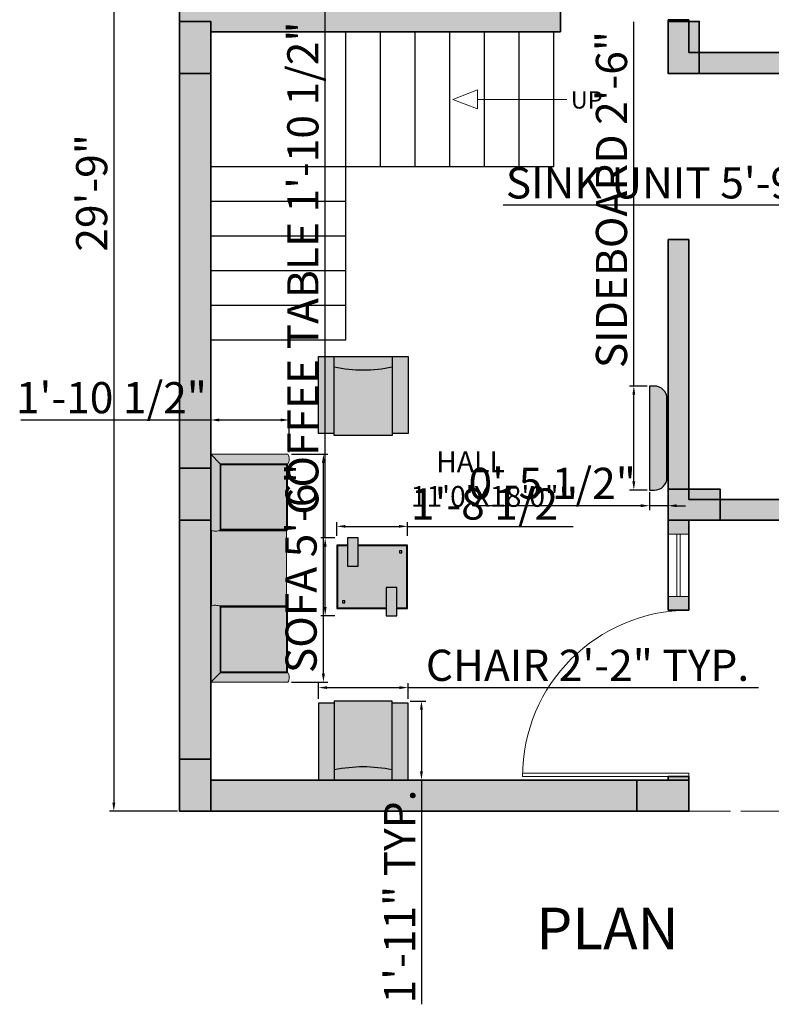
# Model space of a CAD drawing. Units: inches. Extents: x 3148 to 3962, y 1142 to 1671.
# Tile 1 of 9: x 3148 to 3365, y 1142 to 1426. Entities that reach past the tile are written whole.
import ezdxf

# ---------------------------------------------------------------- set-up
doc = ezdxf.new("R2010")
doc.units = ezdxf.units.IN
doc.linetypes.add('ACAD_ISO02W100', pattern=[15, 12, -3])
for name, color, linetype, lineweight in [('A-ANNO-DIMS', 2, 'Continuous', 18), ('A-ANNO-SYMB', 7, 'Continuous', 18), ('A-ANNO-TEXT', 7, 'Continuous', 25), ('A-AREA-IDEN', 7, 'Continuous', 18), ('A-COLS', 1, 'Continuous', 35), ('A-DOOR', 3, 'Continuous', 18), ('A-FLOR-STRS', 7, 'Continuous', 25), ('A-FURN', 8, 'Continuous', 18), ('A-GLAZ', 4, 'Continuous', 18), ('A-ROOF-OVHD', 7, 'ACAD_ISO02W100', 18), ('A-WALL', 7, 'Continuous', 35), ('moveis', 254, 'Continuous', 5), ('parede', 7, 'Continuous', 30)]:
    doc.layers.add(name, color=color, linetype=linetype, lineweight=lineweight)
doc.layers.add('A-WALL-PATT', color=252, linetype='Continuous', lineweight=13, true_color=0x939598)
doc.layers.add('MESA', color=7, linetype='Continuous')
doc.layers.add('MOBIL', color=7, linetype='Continuous')
doc.styles.get("Standard").update_dxf_attribs({"font": 'arial.ttf'})
doc.dimstyles.new('ISO-25', dxfattribs={"dimtxt": 9, "dimasz": 2.5, "dimexe": 1.25, "dimexo": 0.625, "dimtad": 1, "dimdec": 1, "dimlunit": 3, "dimtxsty": 'Standard', "dimcen": 2.5, "dimadec": 0, "dimazin": 0, "dimtfac": 1, "dimtdec": 1, "dimtmove": 0, "dimatfit": 3, "dimfxl": 1, "dimarcsym": 0})

# ---------------------------------------------------------------- blocks, each defined once
blk = doc.blocks.new('Poltrona Zoom Bolis')
at = {"layer": 'moveis'}
h = blk.add_hatch(color=256, dxfattribs=at)
h.set_gradient(color1=(102, 74, 66), color2=(156, 115, 104), one_color=1, tint=0.51)
h.paths.add_polyline_path([(-0.8363, -0.5604, 0.119368), (-0.805, -0.5689), (-0.7999, -0.5689, 0.109048), (-0.7663, -0.5612), (-0.7663, -0.0639), (-0.8363, 0.0061)])
h = blk.add_hatch(color=256, dxfattribs=at)
h.set_gradient(color1=(102, 74, 66), color2=(156, 115, 104), one_color=1, tint=0.51, name='INVCURVED')
h.paths.add_polyline_path([(-0.2778, -0.0639, 0.078404), (-0.2713, -0.0289), (-0.2713, -0.0252, 0.119368), (-0.2798, 0.0061), (-0.8363, 0.0061), (-0.7663, -0.0639)])
h.paths.add_polyline_path([(0.7663, -0.0639), (0.8363, 0.0061), (0.2798, 0.0061, 0.119368), (0.2713, -0.0252), (0.2713, -0.0289, 0.078404), (0.2778, -0.0639)])
h = blk.add_hatch(color=256, dxfattribs=at)
h.set_gradient(color1=(102, 74, 66), color2=(108, 79, 71), one_color=1, tint=0.35, name='CYLINDER')
h.paths.add_polyline_path([(-0.275, 0), (-0.275, -0.0047, -0.090212), (-0.2713, -0.029, -0.057138), (-0.275, -0.0548), (-0.275, -0.55), (0.275, -0.55), (0.275, -0.0548, -0.057138), (0.2713, -0.029, -0.090212), (0.275, -0.0047), (0.275, 0)])
h = blk.add_hatch(color=256, dxfattribs=at)
h.set_gradient(color1=(102, 74, 66), color2=(156, 115, 104), one_color=1, tint=0.51)
h.paths.add_polyline_path([(0.7663, -0.5612, 0.109048), (0.7999, -0.5689), (0.805, -0.5689, 0.119368), (0.8363, -0.5604), (0.8363, 0.0061), (0.7663, -0.0639)])
h = blk.add_hatch(color=256, dxfattribs=at)
h.set_gradient(color1=(102, 74, 66), color2=(96, 70, 62), one_color=1, tint=0.31, name='CYLINDER')
h.paths.add_polyline_path([(-0.7663, -0.0639), (-0.759, -0.0691), (-0.2798, -0.0691, 0.012038), (-0.2778, -0.0639)])
h.paths.add_polyline_path([(-0.759, -0.0691), (-0.7663, -0.0639), (-0.7663, -0.5612, 0.025931), (-0.759, -0.5573)])
h.paths.add_polyline_path([(-0.2804, -0.0691), (-0.2863, -0.0691), (-0.2863, -0.5489), (-0.759, -0.5489), (-0.759, -0.5573), (-0.2804, -0.5573)])
h = blk.add_hatch(color=256, dxfattribs=at)
h.set_gradient(color1=(102, 74, 66), color2=(156, 115, 104), one_color=1, tint=0.51, name='INVCYLINDER')
h.paths.add_polyline_path([(-0.759, -0.0691), (-0.759, -0.5489), (-0.2863, -0.5489), (-0.2863, -0.0691)])
h = blk.add_hatch(color=256, dxfattribs=at)
h.set_gradient(color1=(102, 74, 66), color2=(96, 70, 62), one_color=1, tint=0.31, name='CYLINDER')
h.paths.add_polyline_path([(0.7663, -0.0639), (0.2778, -0.0639, 0.012038), (0.2798, -0.0691), (0.759, -0.0691)])
h = blk.add_hatch(color=256, dxfattribs=at)
h.set_gradient(color1=(102, 74, 66), color2=(96, 70, 62), one_color=1, tint=0.31, name='CYLINDER')
h.paths.add_polyline_path([(0.2863, -0.0691), (0.2804, -0.0691), (0.2804, -0.5573), (0.759, -0.5573), (0.759, -0.5489), (0.2863, -0.5489)])
h = blk.add_hatch(color=256, dxfattribs=at)
h.set_gradient(color1=(102, 74, 66), color2=(156, 115, 104), one_color=1, tint=0.51, name='INVCYLINDER')
h.paths.add_polyline_path([(0.2863, -0.0691), (0.2863, -0.5489), (0.759, -0.5489), (0.759, -0.0691)])
h = blk.add_hatch(color=256, dxfattribs=at)
h.set_gradient(color1=(102, 74, 66), color2=(96, 70, 62), one_color=1, tint=0.31, name='CYLINDER')
h.paths.add_polyline_path([(0.759, -0.5573, 0.025931), (0.7663, -0.5612), (0.7663, -0.0639), (0.759, -0.0691)])
for p, q in [((-0.8363, 0.0061), (-0.8363, -0.5604)), ((-0.8363, 0.0061), (-0.2798, 0.0061)), ((-0.8363, 0.0061), (-0.7663, -0.0639)), ((0.275, 0), (-0.275, 0)), ((-0.275, -0.0047), (-0.275, 0)), ((0.275, -0.0047), (0.275, 0)), ((0.275, -0.0047), (0.275, 0)), ((0.8363, 0.0061), (0.2798, 0.0061)), ((0.8363, 0.0061), (0.7663, -0.0639)), ((0.8363, 0.0061), (0.8363, -0.5604)), ((-0.7663, -0.5612), (-0.7663, -0.0639)), ((-0.7663, -0.0639), (-0.2778, -0.0639)), ((-0.7663, -0.0639), (-0.759, -0.0691)), ((-0.759, -0.5573), (-0.759, -0.0691)), ((-0.759, -0.0691), (-0.2798, -0.0691)), ((-0.2863, -0.5489), (-0.2863, -0.0691)), ((-0.2804, -0.5573), (-0.2804, -0.0691)), ((-0.275, -0.55), (-0.275, -0.0548)), ((-0.2713, -0.0252), (-0.2713, -0.0327)), ((-0.2713, -0.0327), (-0.2713, -0.0252)), ((0.2713, -0.0252), (0.2713, -0.0327)), ((0.2713, -0.0327), (0.2713, -0.0252)), ((0.275, -0.55), (0.275, -0.0548)), ((0.7663, -0.0639), (0.2778, -0.0639)), ((0.759, -0.0691), (0.2798, -0.0691)), ((0.2804, -0.5573), (0.2804, -0.0691)), ((0.2863, -0.5489), (0.2863, -0.0691)), ((0.7663, -0.0639), (0.759, -0.0691)), ((0.759, -0.5573), (0.759, -0.0691)), ((0.7663, -0.5612), (0.7663, -0.0639)), ((-0.805, -0.5689), (-0.7975, -0.5689)), ((-0.759, -0.5489), (-0.2863, -0.5489)), ((-0.759, -0.5573), (-0.2804, -0.5573)), ((-0.275, -0.55), (0.275, -0.55)), ((0.759, -0.5573), (0.2804, -0.5573)), ((0.759, -0.5489), (0.2863, -0.5489)), ((0.805, -0.5689), (0.7975, -0.5689))]:
    blk.add_line(p, q, dxfattribs=at)
for centre, radius, start, end in [((-0.3401, -0.0271), 0.0688, 358.44064, 28.78774), ((0.3401, -0.0271), 0.0688, 151.21226, 181.55936), ((-0.3855, -0.0258), 0.1142, 337.7295, 358.42044), ((0.3855, -0.0258), 0.1142, 181.57956, 202.2705), ((-0.8032, -0.5002), 0.0688, 241.21226, 271.55936), ((-0.8006, -0.4888), 0.0801, 269.51513, 301.32015), ((0.8006, -0.4888), 0.0801, 238.67985, 270.48487), ((0.8032, -0.5002), 0.0688, 268.44064, 298.78774)]:
    blk.add_arc(centre, radius, start, end, dxfattribs=at)
blk = doc.blocks.new('Buffet 2.49x0.42 Imbuia')
at = {"layer": 'MOBIL', "ltscale": 0.02}
h = blk.add_hatch(color=256, dxfattribs=at)
h.set_gradient(color1=(96, 70, 47), color2=(44, 32, 22), one_color=1, tint=0.13, name='INVCURVED')
h.paths.add_polyline_path([(-1.245, 0), (-1.245, -0.12, 0.414214), (-0.945, -0.42), (0.945, -0.42, 0.414214), (1.245, -0.12), (1.245, 0)])
h = blk.add_hatch(color=256, dxfattribs=at)
h.set_gradient(color1=(162, 174, 173), one_color=1, tint=1, name='CURVED')
h.paths.add_polyline_path([(-0.483, -0.435, -0.362573), (-0.481, -0.43), (-0.5, -0.43, -0.362573), (-0.499, -0.435, 0.47966), (-0.491, -0.446, 0.47966)])
h = blk.add_hatch(color=256, dxfattribs=at)
h.set_gradient(color1=(162, 174, 173), one_color=1, tint=1, name='CURVED')
h.paths.add_polyline_path([(0.008, -0.435, -0.362573), (0.01, -0.43), (-0.01, -0.43, -0.362573), (-0.008, -0.435, 0.47966), (0, -0.446, 0.47966)])
h = blk.add_hatch(color=256, dxfattribs=at)
h.set_gradient(color1=(162, 174, 173), one_color=1, tint=1, name='CURVED')
h.paths.add_polyline_path([(0.499, -0.435, -0.362573), (0.5, -0.43), (0.481, -0.43, -0.362573), (0.483, -0.435, 0.47966), (0.491, -0.446, 0.47966)])
blk.add_lwpolyline([(-0.945, -0.42), (0.945, -0.42, 0.414214), (1.245, -0.12), (1.245, 0), (-1.245, 0), (-1.245, -0.12, 0.414214)], format="xyb", close=True, dxfattribs=at)
for points in [[(-0.726, -0.43), (-0.256, -0.43), (-0.256, -0.42), (-0.726, -0.42)], [(-0.235, -0.43), (0.235, -0.43), (0.235, -0.42), (-0.235, -0.42)], [(0.726, -0.43), (0.256, -0.43), (0.256, -0.42), (0.726, -0.42)]]:
    blk.add_lwpolyline(points, close=True, dxfattribs=at)
for centre, radius, start, end in [((-0.503, -0.433), 0.00412, 338.2249, 57.942), ((-0.49, -0.437), 0.00871, 165.3691, 267.8698), ((-0.491, -0.432), 0.00985, 233.2504, 306.7496), ((-0.491, -0.437), 0.00871, 272.1302, 14.6309), ((-0.479, -0.433), 0.00412, 122.058, 201.7751), ((-0.012, -0.433), 0.00412, 338.2249, 57.942), ((0, -0.437), 0.00871, 165.3691, 267.8698), ((0, -0.432), 0.00985, 233.2504, 306.7496), ((0, -0.437), 0.00871, 272.1302, 14.6309), ((0.012, -0.433), 0.00412, 122.058, 201.7751), ((0.479, -0.433), 0.00412, 338.2249, 57.942), ((0.491, -0.437), 0.00871, 165.3691, 267.8698), ((0.491, -0.432), 0.00985, 233.2504, 306.7496), ((0.49, -0.437), 0.00871, 272.1302, 14.6309), ((0.503, -0.433), 0.00412, 122.058, 201.7751)]:
    blk.add_arc(centre, radius, start, end, dxfattribs=at)
blk = doc.blocks.new('Polt. Palla - Marrom')
at = {"layer": 'parede', "ltscale": 0.8}
h = blk.add_hatch(color=256, dxfattribs=at)
h.set_gradient(color1=(96, 64, 57), color2=(150, 101, 90), one_color=1, tint=0.47, name='CYLINDER')
h.paths.add_polyline_path([(-0.425, -0.7313), (-0.275, -0.7313), (-0.275, 0), (-0.425, 0)])
h = blk.add_hatch(color=256, dxfattribs=at)
h.set_gradient(color1=(96, 64, 57), color2=(150, 101, 90), one_color=1, tint=0.47, name='CURVED')
h.paths.add_polyline_path([(0.275, -0.0986), (0.275, 0), (-0.275, 0), (-0.275, -0.0986, 0.10456)])
h = blk.add_hatch(color=256, dxfattribs=at)
h.set_gradient(color1=(96, 64, 57), color2=(150, 101, 90), one_color=1, tint=0.47, name='CYLINDER')
h.paths.add_polyline_path([(0.425, 0), (0.275, 0), (0.275, -0.7313), (0.425, -0.7313)])
h = blk.add_hatch(color=256, dxfattribs=at)
h.set_gradient(color1=(96, 64, 57), color2=(150, 101, 90), one_color=1, tint=0.47, name='INVCURVED')
h.paths.add_polyline_path([(0.275, -0.0986, -0.10456), (-0.275, -0.0986), (-0.275, -0.75), (0.275, -0.75)])
at = {"layer": 'MESA'}
for p, q in [((-0.425, 0), (0.425, 0)), ((-0.425, -0.7313), (-0.425, 0)), ((-0.275, -0.75), (-0.275, 0)), ((0.275, 0), (0.275, -0.75)), ((0.425, 0), (0.425, -0.7313)), ((-0.275, -0.7313), (-0.425, -0.7313)), ((0.425, -0.7313), (0.275, -0.7313)), ((0.275, -0.75), (-0.275, -0.75))]:
    blk.add_line(p, q, dxfattribs=at)
blk.add_arc((0, 1.202), 1.3294, 258.06163, 281.93837, dxfattribs=at)
blk = doc.blocks.new('Mesa de centro Cantria feeling')
at = {"layer": 'MOBIL', "ltscale": 0.2}
h = blk.add_hatch(color=256, dxfattribs=at)
h.set_gradient(color1=(74, 55, 38), color2=(104, 77, 54), one_color=1, tint=0.31, name='CYLINDER')
h.paths.add_polyline_path([(-0.85, -0.3), (-0.7, -0.3), (-0.7, 0.1), (-0.85, 0.1)])
h = blk.add_hatch(color=256, dxfattribs=at)
h.set_gradient(color1=(221, 221, 223), one_color=1, tint=1)
h.paths.add_polyline_path([(-0.15, -0.6), (-0.15, -0.89), (-0.01, -0.89), (-0.01, -0.01), (-0.7, -0.01), (-0.7, -0.3), (-0.85, -0.3), (-0.85, -0.01), (-0.99, -0.01), (-0.99, -0.89), (-0.3, -0.89), (-0.3, -0.6)])
h.paths.add_polyline_path([(-0.112, -0.112), (-0.112, -0.082), (-0.082, -0.082), (-0.082, -0.112)], flags=16)
h.paths.add_polyline_path([(-0.888, -0.788), (-0.888, -0.818), (-0.918, -0.818), (-0.918, -0.788)], flags=16)
h = blk.add_hatch(color=256, dxfattribs=at)
h.set_gradient(color1=(74, 55, 38), color2=(104, 77, 54), one_color=1, tint=0.31, name='CYLINDER')
h.paths.add_polyline_path([(-0.15, -0.6), (-0.3, -0.6), (-0.3, -1), (-0.15, -1)])
for points in [[(-0.85, 0), (-1, 0), (-1, -0.9), (-0.3, -0.9)], [(-0.15, -0.9), (0, -0.9), (0, 0), (-0.7, 0)], [(-0.85, -0.01), (-0.99, -0.01), (-0.99, -0.89), (-0.3, -0.89)], [(-0.15, -0.89), (-0.01, -0.89), (-0.01, -0.01), (-0.7, -0.01)]]:
    blk.add_lwpolyline(points, dxfattribs=at)
for points in [[(-0.85, -0.3), (-0.7, -0.3), (-0.7, 0.1), (-0.85, 0.1)], [(-0.082, -0.082), (-0.112, -0.082), (-0.112, -0.112), (-0.082, -0.112)], [(-0.15, -0.6), (-0.3, -0.6), (-0.3, -1), (-0.15, -1)], [(-0.918, -0.818), (-0.888, -0.818), (-0.888, -0.788), (-0.918, -0.788)]]:
    blk.add_lwpolyline(points, close=True, dxfattribs=at)
blk = doc.blocks.new('*D43')
at = {"layer": 'A-ANNO-DIMS', "color": 0, "lineweight": -2, "transparency": 16777216}
for p, q in [((3193.42, 1554.8), (3173.83, 1554.8)), ((3175.08, 1552.3), (3175.08, 1200.3)), ((3193.42, 1197.8), (3173.83, 1197.8))]:
    blk.add_line(p, q, dxfattribs=at)
at = {"layer": 'A-ANNO-DIMS', "color": 0, "transparency": 16777216}
for points in [[(3174.66, 1552.3), (3175.5, 1552.3), (3175.08, 1554.8)], [(3174.66, 1200.3), (3175.5, 1200.3), (3175.08, 1197.8)]]:
    blk.add_solid(points, dxfattribs=at)
at = {"layer": 'Defpoints', "color": 0, "transparency": 16777216}
for p in [(3194.04, 1554.8), (3175.08, 1197.8), (3194.04, 1197.8)]:
    blk.add_point(p, dxfattribs=at)
at = {"layer": 'A-ANNO-DIMS', "color": 0, "transparency": 16777216, "insert": (3169.86, 1376.3), "char_height": 9, "attachment_point": 5, "rotation": 90}
blk.add_mtext('29\'-9"', dxfattribs=at)
blk = doc.blocks.new('DOOR-SWING-48')
for p, q in [((-48, 0), (0, 0)), ((-47.99, 1), (0, 1)), ((0, 0), (0, 1))]:
    blk.add_line(p, q)
blk.add_arc((0, 0), 48, 90, 180)
blk = doc.blocks.new('WIN-18')
for p, q in [((0, 18), (6, 18)), ((2.5, 0), (2.5, 18)), ((3.5, 0), (3.5, 18)), ((0, 0), (6, 0))]:
    blk.add_line(p, q)
blk = doc.blocks.new('STAIR-QUARTER-TURN')
for p, q in [((39, 0), (39, 89)), ((49, 50), (49, 89)), ((59, 50), (59, 89)), ((69, 50), (69, 89)), ((79, 50), (79, 89)), ((89, 50), (89, 89)), ((99, 50), (99, 89)), ((99, 50), (0, 50)), ((39, 40), (0, 40)), ((39, 30), (0, 30)), ((39, 20), (0, 20)), ((39, 10), (0, 10)), ((39, 0), (0, 0))]:
    blk.add_line(p, q)
blk = doc.blocks.new('COL-9X15')
h = blk.add_hatch(color=256)
h.dxf.hatch_style = 1
h.paths.add_polyline_path([(9, 15), (0, 15), (0, 0), (9, 0)])
blk.add_lwpolyline([(9, 0), (9, 15), (0, 15), (0, 0)], close=True)
blk = doc.blocks.new('STAIR-UP-ARROW')
blk.add_line((32.89, 2.71), (7.09, 2.71))
blk.add_lwpolyline([(0, 2.71), (7.09, 0), (7.09, 5.42)], close=True)
blk.add_text('UP', height=5).set_placement((33.98, 0.05))
blk = doc.blocks.new('*D88')
at = {"layer": 'A-ANNO-DIMS', "color": 0, "lineweight": -2, "transparency": 16777216}
for p, q in [((3234.15, 1230.22), (3234.15, 1234.72)), ((3259.99, 1230.22), (3259.99, 1234.72)), ((3236.65, 1233.47), (3257.49, 1233.47)), ((3259.99, 1233.47), (3361.1, 1233.47))]:
    blk.add_line(p, q, dxfattribs=at)
at = {"layer": 'A-ANNO-DIMS', "color": 0, "transparency": 16777216}
for points in [[(3236.65, 1233.89), (3236.65, 1233.06), (3234.15, 1233.47)], [(3257.49, 1233.89), (3257.49, 1233.06), (3259.99, 1233.47)]]:
    blk.add_solid(points, dxfattribs=at)
at = {"layer": 'Defpoints', "color": 0, "transparency": 16777216}
for p in [(3259.99, 1233.47), (3234.15, 1229.6), (3259.99, 1229.6)]:
    blk.add_point(p, dxfattribs=at)
at = {"layer": 'A-ANNO-DIMS', "color": 0, "transparency": 16777216, "insert": (3311.8, 1238.75), "char_height": 9, "attachment_point": 5}
blk.add_mtext('CHAIR 2\'-2" TYP.', dxfattribs=at)
blk = doc.blocks.new('*D89')
at = {"layer": 'A-ANNO-DIMS', "color": 0, "lineweight": -2, "transparency": 16777216}
for p, q in [((3260.61, 1229.6), (3265.11, 1229.6)), ((3263.86, 1227.1), (3263.86, 1209.3)), ((3260.61, 1206.8), (3265.11, 1206.8)), ((3263.86, 1206.8), (3263.86, 1142.04))]:
    blk.add_line(p, q, dxfattribs=at)
at = {"layer": 'A-ANNO-DIMS', "color": 0, "transparency": 16777216}
for points in [[(3263.45, 1227.1), (3264.28, 1227.1), (3263.86, 1229.6)], [(3263.45, 1209.3), (3264.28, 1209.3), (3263.86, 1206.8)]]:
    blk.add_solid(points, dxfattribs=at)
at = {"layer": 'Defpoints', "color": 0, "transparency": 16777216}
for p in [(3259.99, 1229.6), (3259.99, 1206.8), (3263.86, 1206.8)]:
    blk.add_point(p, dxfattribs=at)
at = {"layer": 'A-ANNO-DIMS', "color": 0, "transparency": 16777216, "insert": (3258.72, 1173.17), "char_height": 9, "attachment_point": 5, "rotation": 90}
blk.add_mtext('1\'-11" TYP.', dxfattribs=at)
blk = doc.blocks.new('*D96')
at = {"layer": 'A-ANNO-DIMS', "color": 0, "lineweight": -2, "transparency": 16777216}
for p, q in [((3383.35, 1376.46), (3383.35, 1500.1)), ((3390.32, 1376.46), (3382.1, 1376.46)), ((3383.35, 1328.3), (3383.35, 1373.96)), ((3390.32, 1325.8), (3382.1, 1325.8))]:
    blk.add_line(p, q, dxfattribs=at)
at = {"layer": 'A-ANNO-DIMS', "color": 0, "transparency": 16777216}
for points in [[(3382.93, 1373.96), (3383.77, 1373.96), (3383.35, 1376.46)], [(3382.93, 1328.3), (3383.77, 1328.3), (3383.35, 1325.8)]]:
    blk.add_solid(points, dxfattribs=at)
at = {"layer": 'Defpoints', "color": 0, "transparency": 16777216}
for p in [(3383.35, 1376.46), (3390.95, 1376.46), (3390.95, 1325.8)]:
    blk.add_point(p, dxfattribs=at)
at = {"layer": 'A-ANNO-DIMS', "color": 0, "transparency": 16777216, "insert": (3378.07, 1439.53), "char_height": 9, "attachment_point": 5, "rotation": 90}
blk.add_mtext('DINING SET 4\'-2 1/2"', dxfattribs=at)
blk = doc.blocks.new('*D98')
at = {"layer": 'A-ANNO-DIMS', "color": 0, "lineweight": -2, "transparency": 16777216}
for p, q in [((3226.32, 1300.86), (3236.82, 1300.86)), ((3235.57, 1237.51), (3235.57, 1298.36)), ((3226.32, 1235.01), (3236.82, 1235.01))]:
    blk.add_line(p, q, dxfattribs=at)
at = {"layer": 'A-ANNO-DIMS', "color": 0, "transparency": 16777216}
for points in [[(3235.15, 1298.36), (3235.99, 1298.36), (3235.57, 1300.86)], [(3235.15, 1237.51), (3235.99, 1237.51), (3235.57, 1235.01)]]:
    blk.add_solid(points, dxfattribs=at)
at = {"layer": 'Defpoints', "color": 0, "transparency": 16777216}
for p in [(3225.69, 1300.86), (3235.57, 1300.86), (3225.69, 1235.01)]:
    blk.add_point(p, dxfattribs=at)
at = {"layer": 'A-ANNO-DIMS', "color": 0, "transparency": 16777216, "insert": (3230.29, 1267.93), "char_height": 9, "attachment_point": 5, "rotation": 90}
blk.add_mtext('SOFA 5\'-6"', dxfattribs=at)
blk = doc.blocks.new('*D99')
at = {"layer": 'A-ANNO-DIMS', "color": 0, "lineweight": -2, "transparency": 16777216}
for p, q in [((3203.04, 1310.73), (3148.25, 1310.73)), ((3203.04, 1301.48), (3203.04, 1311.98)), ((3223.19, 1310.73), (3205.54, 1310.73)), ((3225.69, 1301.48), (3225.69, 1311.98))]:
    blk.add_line(p, q, dxfattribs=at)
at = {"layer": 'A-ANNO-DIMS', "color": 0, "transparency": 16777216}
for points in [[(3205.54, 1311.15), (3205.54, 1310.32), (3203.04, 1310.73)], [(3223.19, 1311.15), (3223.19, 1310.32), (3225.69, 1310.73)]]:
    blk.add_solid(points, dxfattribs=at)
at = {"layer": 'Defpoints', "color": 0, "transparency": 16777216}
for p in [(3203.04, 1310.73), (3203.04, 1300.86), (3225.69, 1300.86)]:
    blk.add_point(p, dxfattribs=at)
at = {"layer": 'A-ANNO-DIMS', "color": 0, "transparency": 16777216, "insert": (3174.4, 1316.01), "char_height": 9, "attachment_point": 5}
blk.add_mtext('1\'-10 1/2"', dxfattribs=at)
blk = doc.blocks.new('*D100')
at = {"layer": 'A-ANNO-DIMS', "color": 0, "lineweight": -2, "transparency": 16777216}
for p, q in [((3325.16, 1320.53), (3325.16, 1425.71)), ((3329.04, 1320.53), (3323.91, 1320.53)), ((3325.16, 1293), (3325.16, 1318.03)), ((3329.04, 1290.5), (3323.91, 1290.5))]:
    blk.add_line(p, q, dxfattribs=at)
at = {"layer": 'A-ANNO-DIMS', "color": 0, "transparency": 16777216}
for points in [[(3324.74, 1318.03), (3325.57, 1318.03), (3325.16, 1320.53)], [(3324.74, 1293), (3325.57, 1293), (3325.16, 1290.5)]]:
    blk.add_solid(points, dxfattribs=at)
at = {"layer": 'Defpoints', "color": 0, "transparency": 16777216}
for p in [(3325.16, 1320.53), (3329.66, 1320.53), (3329.66, 1290.5)]:
    blk.add_point(p, dxfattribs=at)
at = {"layer": 'A-ANNO-DIMS', "color": 0, "transparency": 16777216, "insert": (3319.88, 1374.37), "char_height": 9, "attachment_point": 5, "rotation": 90}
blk.add_mtext('SIDEBOARD 2\'-6"', dxfattribs=at)
blk = doc.blocks.new('*D101')
at = {"layer": 'A-ANNO-DIMS', "color": 0, "lineweight": -2, "transparency": 16777216}
for p, q in [((3329.66, 1289.87), (3329.66, 1284.74)), ((3335.04, 1289.87), (3335.04, 1284.74)), ((3327.16, 1285.99), (3278.52, 1285.99)), ((3335.04, 1285.99), (3329.66, 1285.99)), ((3337.54, 1285.99), (3340.04, 1285.99))]:
    blk.add_line(p, q, dxfattribs=at)
at = {"layer": 'A-ANNO-DIMS', "color": 0, "transparency": 16777216}
for points in [[(3327.16, 1286.41), (3327.16, 1285.57), (3329.66, 1285.99)], [(3337.54, 1286.41), (3337.54, 1285.57), (3335.04, 1285.99)]]:
    blk.add_solid(points, dxfattribs=at)
at = {"layer": 'Defpoints', "color": 0, "transparency": 16777216}
for p in [(3329.66, 1290.5), (3335.04, 1290.5), (3329.66, 1285.99)]:
    blk.add_point(p, dxfattribs=at)
at = {"layer": 'A-ANNO-DIMS', "color": 0, "transparency": 16777216, "insert": (3301.59, 1291.27), "char_height": 9, "attachment_point": 5}
blk.add_mtext('0\'-5 1/2"', dxfattribs=at)
blk = doc.blocks.new('*D102')
at = {"layer": 'A-ANNO-DIMS', "color": 0, "lineweight": -2, "transparency": 16777216}
for p, q in [((3236.08, 1276.67), (3236.08, 1430.01)), ((3238.82, 1276.67), (3234.83, 1276.67)), ((3236.08, 1256.73), (3236.08, 1274.17)), ((3238.82, 1254.23), (3234.83, 1254.23))]:
    blk.add_line(p, q, dxfattribs=at)
at = {"layer": 'A-ANNO-DIMS', "color": 0, "transparency": 16777216}
for points in [[(3235.66, 1274.17), (3236.49, 1274.17), (3236.08, 1276.67)], [(3235.66, 1256.73), (3236.49, 1256.73), (3236.08, 1254.23)]]:
    blk.add_solid(points, dxfattribs=at)
at = {"layer": 'Defpoints', "color": 0, "transparency": 16777216}
for p in [(3236.08, 1276.67), (3239.44, 1276.67), (3239.44, 1254.23)]:
    blk.add_point(p, dxfattribs=at)
at = {"layer": 'A-ANNO-DIMS', "color": 0, "transparency": 16777216, "insert": (3230.8, 1354.59), "char_height": 9, "attachment_point": 5, "rotation": 90}
blk.add_mtext('COFFEE TABLE 1\'-10 1/2"', dxfattribs=at)
blk = doc.blocks.new('*D103')
at = {"layer": 'A-ANNO-DIMS', "color": 0, "lineweight": -2, "transparency": 16777216}
for p, q in [((3239.44, 1277.29), (3239.44, 1281.28)), ((3241.94, 1280.03), (3257.34, 1280.03)), ((3259.84, 1277.29), (3259.84, 1281.28)), ((3259.84, 1280.03), (3307.64, 1280.03))]:
    blk.add_line(p, q, dxfattribs=at)
at = {"layer": 'A-ANNO-DIMS', "color": 0, "transparency": 16777216}
for points in [[(3241.94, 1280.45), (3241.94, 1279.62), (3239.44, 1280.03)], [(3257.34, 1280.45), (3257.34, 1279.62), (3259.84, 1280.03)]]:
    blk.add_solid(points, dxfattribs=at)
at = {"layer": 'Defpoints', "color": 0, "transparency": 16777216}
for p in [(3259.84, 1280.03), (3239.44, 1276.67), (3259.84, 1276.67)]:
    blk.add_point(p, dxfattribs=at)
at = {"layer": 'A-ANNO-DIMS', "color": 0, "transparency": 16777216, "insert": (3284.99, 1285.31), "char_height": 9, "attachment_point": 5}
blk.add_mtext('1\'-8 1/2"', dxfattribs=at)
blk = doc.blocks.new('*D108')
at = {"layer": 'A-ANNO-DIMS', "color": 0, "lineweight": -2, "transparency": 16777216}
for p, q in [((3401.7, 1382.52), (3401.7, 1371.49)), ((3471.03, 1382.52), (3471.03, 1371.49)), ((3401.7, 1372.74), (3287.44, 1372.74)), ((3468.53, 1372.74), (3404.2, 1372.74))]:
    blk.add_line(p, q, dxfattribs=at)
at = {"layer": 'A-ANNO-DIMS', "color": 0, "transparency": 16777216}
for points in [[(3404.2, 1373.16), (3404.2, 1372.33), (3401.7, 1372.74)], [(3468.53, 1373.16), (3468.53, 1372.33), (3471.03, 1372.74)]]:
    blk.add_solid(points, dxfattribs=at)
at = {"layer": 'Defpoints', "color": 0, "transparency": 16777216}
for p in [(3401.7, 1383.14), (3471.03, 1383.14), (3401.7, 1372.74)]:
    blk.add_point(p, dxfattribs=at)
at = {"layer": 'A-ANNO-DIMS', "color": 0, "transparency": 16777216, "insert": (3343.32, 1378.02), "char_height": 9, "attachment_point": 5}
blk.add_mtext('SINK UNIT 5\'-9 1/2"', dxfattribs=at)

msp = doc.modelspace()

# ---------------------------------------------------------------- hatches: boundary and pattern name
at = {"layer": 'A-WALL-PATT'}
h = msp.add_hatch(color=256, dxfattribs=at)
h.dxf.hatch_style = 1
h.paths.add_polyline_path([(3203.04, 1410.8), (3194.04, 1410.8), (3194.04, 1296.8), (3203.04, 1296.8), (3203.04, 1300.86)])
h.paths.add_polyline_path([(3203.04, 1281.8), (3194.04, 1281.8), (3194.04, 1212.8), (3203.04, 1212.8)])
h.paths.add_polyline_path([(3326.04, 1206.8), (3203.04, 1206.8), (3203.04, 1197.8), (3326.04, 1197.8)])
h.paths.add_polyline_path([(3341.04, 1362.8), (3335.04, 1362.8), (3335.04, 1290.8), (3341.04, 1290.8)])
h.paths.add_polyline_path([(3341.04, 1207.8), (3335.04, 1207.8), (3335.04, 1206.8), (3341.04, 1206.8)])
h.paths.add_polyline_path([(3341.04, 1259.8), (3335.04, 1259.8), (3335.04, 1255.8), (3341.04, 1255.8)])
h.paths.add_polyline_path([(3341.04, 1281.8), (3335.04, 1281.8), (3335.04, 1277.8), (3341.04, 1277.8)])
h.paths.add_polyline_path([(3377.04, 1287.8), (3350.04, 1287.8), (3350.04, 1281.8), (3377.04, 1281.8)])
h.paths.add_polyline_path([(3473.04, 1287.8), (3445.04, 1287.8), (3437.04, 1287.8), (3437.04, 1281.8), (3473.04, 1281.8)])
h.paths.add_polyline_path([(3482.04, 1313.3), (3473.04, 1313.3), (3473.04, 1296.8), (3482.04, 1296.8)])
h.paths.add_polyline_path([(3482.04, 1410.8), (3473.04, 1410.8), (3473.04, 1385.3), (3482.04, 1385.3)])
h.paths.add_polyline_path([(3473.04, 1416.8), (3344.04, 1416.8), (3344.04, 1410.8), (3473.04, 1410.8)])
h.paths.add_polyline_path([(3482.04, 1445.3), (3473.04, 1445.3), (3473.04, 1425.8), (3482.04, 1425.8)])
h.paths.add_polyline_path([(3341.04, 1426.3), (3335.04, 1426.3), (3335.04, 1425.8), (3341.04, 1425.8)])
h.paths.add_polyline_path([(3304.04, 1428.8), (3253.54, 1428.8), (3253.54, 1430.3), (3251.04, 1430.3), (3251.04, 1428.8), (3203.04, 1428.8), (3203.04, 1512.8), (3215.04, 1512.8), (3215.04, 1518.8), (3203.04, 1518.8), (3203.04, 1539.8), (3194.04, 1539.8), (3194.04, 1425.8), (3203.04, 1425.8), (3203.04, 1422.8), (3304.04, 1422.8)])
h.paths.add_polyline_path([(3265.54, 1518.8), (3239.04, 1518.8), (3239.04, 1512.8), (3251.04, 1512.8), (3251.04, 1461.3), (3253.54, 1461.3), (3253.54, 1462.3), (3255.54, 1462.3), (3255.54, 1464.8), (3253.54, 1464.8), (3253.54, 1512.8), (3265.54, 1512.8)], flags=17)
h.paths.add_polyline_path([(3307.54, 1518.8), (3289.54, 1518.8), (3289.54, 1512.8), (3301.54, 1512.8), (3301.54, 1464.8), (3286.54, 1464.8), (3286.54, 1462.3), (3304.04, 1462.3), (3304.04, 1512.8), (3307.54, 1512.8)])
h.paths.add_polyline_path([(3341.04, 1539.8), (3335.04, 1539.8), (3335.04, 1518.8), (3331.54, 1518.8), (3331.54, 1512.8), (3335.04, 1512.8), (3335.04, 1462.3), (3341.04, 1462.3)])
h.paths.add_polyline_path([(3335.04, 1554.8), (3203.04, 1554.8), (3203.04, 1545.8), (3335.04, 1545.8)])
h.paths.add_polyline_path([(3473.04, 1554.8), (3344.04, 1554.8), (3344.04, 1545.8), (3362.94, 1545.8), (3473.04, 1545.8)])
h.paths.add_polyline_path([(3482.04, 1539.8), (3473.04, 1539.8), (3473.04, 1517.3), (3482.04, 1517.3)])

# ---------------------------------------------------------------- linework, layer by layer
at = {"layer": 'A-ROOF-OVHD'}
msp.add_line((3341.04, 1197.8), (3482.04, 1197.8), dxfattribs=at)
at = {"layer": 'A-WALL'}
for p, q in [((3194.04, 1197.8), (3194.04, 1554.8)), ((3304.04, 1422.8), (3304.04, 1428.8)), ((3335.04, 1426.3), (3341.04, 1426.3)), ((3335.04, 1426.3), (3335.04, 1410.8)), ((3341.04, 1426.3), (3341.04, 1416.8)), ((3203.04, 1206.8), (3203.04, 1422.8)), ((3304.04, 1422.8), (3203.04, 1422.8)), ((3473.04, 1416.8), (3341.04, 1416.8)), ((3473.04, 1410.8), (3335.04, 1410.8)), ((3341.04, 1362.8), (3335.04, 1362.8)), ((3335.04, 1362.8), (3335.04, 1255.8)), ((3341.04, 1362.8), (3341.04, 1287.8)), ((3341.04, 1287.8), (3473.04, 1287.8)), ((3341.04, 1281.8), (3473.04, 1281.8)), ((3341.04, 1281.8), (3341.04, 1255.8)), ((3341.04, 1255.8), (3335.04, 1255.8)), ((3341.04, 1206.8), (3203.04, 1206.8)), ((3341.04, 1207.8), (3335.04, 1207.8)), ((3335.04, 1207.8), (3335.04, 1206.8)), ((3341.04, 1207.8), (3341.04, 1206.8)), ((3341.04, 1206.8), (3341.04, 1197.8)), ((3341.04, 1197.8), (3194.04, 1197.8))]:
    msp.add_line(p, q, dxfattribs=at)

# ---------------------------------------------------------------- block references
at = {"layer": 'A-ANNO-SYMB'}
msp.add_blockref('STAIR-UP-ARROW', (3272.97, 1400.59), dxfattribs=at)
at = {"layer": 'A-COLS'}
for p in [(3194.04, 1410.8), (3335.04, 1410.8), (3194.04, 1281.8), (3194.04, 1197.8)]:
    msp.add_blockref('COL-9X15', p, dxfattribs=at)
for p, rotation in [((3335.04, 1290.8), 269.9999999999962), ((3326.04, 1206.8), 269.999999999999)]:
    msp.add_blockref('COL-9X15', p, dxfattribs=dict(at, rotation=rotation))
at = {"layer": 'A-DOOR'}
msp.add_blockref('DOOR-SWING-48', (3341.04, 1207.8), dxfattribs=at)
at = {"layer": 'A-FLOR-STRS'}
msp.add_blockref('STAIR-QUARTER-TURN', (3203.04, 1333.8), dxfattribs=at)
at = {"layer": 'A-FURN'}
for name, p, xscale, yscale, zscale in [('Polt. Palla - Marrom', (3247.07, 1329.06), 30.39650519951174, 30.39650519951174, 30.39650519951174), ('Mesa de centro Cantria feeling', (3259.84, 1274.63), 20.39495612910847, 20.39495612910847, 20.39495612910847)]:
    msp.add_blockref(name, p, dxfattribs=dict(at, xscale=xscale, yscale=yscale, zscale=zscale))
for name, p, xscale, yscale, zscale, rotation in [('Buffet 2.49x0.42 Imbuia', (3329.66, 1305.51), 12.06253257204141, 12.06253257204141, 12.06253257204141, 89.99999999999999), ('Poltrona Zoom Bolis', (3203.28, 1267.93), 39.3701, 39.3701, 39.3701, 89.99999999998717), ('Polt. Palla - Marrom', (3247.07, 1206.8), -30.39650519951174, 30.39650519951174, 30.39650519951174, 180)]:
    msp.add_blockref(name, p, dxfattribs=dict(at, xscale=xscale, yscale=yscale, zscale=zscale, rotation=rotation))
at = {"layer": 'A-GLAZ', "rotation": 180}
msp.add_blockref('WIN-18', (3341.04, 1277.8), dxfattribs=at)

# ---------------------------------------------------------------- texts
at = {"layer": 'A-ANNO-TEXT', "insert": (3297.05, 1169.94), "char_height": 12, "attachment_point": 1}
msp.add_mtext_dynamic_manual_height_columns('PLAN', width=77.9518, gutter_width=12.5, heights=[0], dxfattribs=at)
at = {"layer": 'A-AREA-IDEN', "insert": (3260.76, 1301.67), "char_height": 6, "attachment_point": 1}
msp.add_mtext_dynamic_manual_height_columns('    HALL\\P11\'0\'X18\'0"', width=77.9518, gutter_width=12.5, heights=[0], dxfattribs=at)

# ---------------------------------------------------------------- dimensions: what is measured, and where the dimension line sits
at = {"layer": 'A-ANNO-DIMS'}
for base, p1, p2, angle, override, picture, middle in [((3175.08, 1197.8), (3194.04, 1554.8), (3194.04, 1197.8), 90, {"dimclrd": 0, "dimclre": 0, "dimclrt": 0}, '*D43', (3169.86, 1376.3)), ((3203.0423, 1310.7329), (3225.6932, 1300.8554), (3203.0423, 1300.8554), 180, {"dimdec": 1, "dimlfac": 1, "dimrnd": 0, "dimzin": 1, "dimdsep": 46, "dimlunit": 4, "dimfrac": 2}, '*D99', (3174.3968, 1316.0114)), ((3329.66, 1285.99), (3335.04, 1290.5), (3329.66, 1290.5), 180, {"dimdec": 1, "dimlfac": 1, "dimrnd": 0, "dimzin": 1, "dimdsep": 46, "dimlunit": 4, "dimfrac": 2}, '*D101', (3301.59, 1291.27))]:
    dim = msp.add_linear_dim(base=base, p1=p1, p2=p2, angle=angle, dimstyle='ISO-25', override=override, dxfattribs=at)
    dim.commit()
    dim.dimension.update_dxf_attribs({"geometry": picture, "text_midpoint": middle})
for base, p1, p2, angle, text, picture, middle in [((3383.35, 1376.46), (3390.95, 1325.8), (3390.95, 1376.46), 90, 'DINING SET <>', '*D96', (3378.07, 1439.53)), ((3236.08, 1276.67), (3239.44, 1254.23), (3239.44, 1276.67), 90, 'COFFEE TABLE <>', '*D102', (3230.8, 1354.59)), ((3325.16, 1320.53), (3329.66, 1290.5), (3329.66, 1320.53), 90, 'SIDEBOARD <>', '*D100', (3319.88, 1374.37)), ((3401.7, 1372.74), (3471.03, 1383.14), (3401.7, 1383.14), 180, 'SINK UNIT <>', '*D108', (3343.32, 1378.02)), ((3235.57069, 1300.85538), (3225.6932, 1235.00543), (3225.6932, 1300.85538), 90, 'SOFA <>', '*D98', (3230.28915, 1267.93041)), ((3263.86, 1206.8), (3259.99, 1229.6), (3259.99, 1206.8), 270, '<> TYP.', '*D89', (3258.72, 1173.17))]:
    dim = msp.add_linear_dim(base=base, p1=p1, p2=p2, angle=angle, text=text, dimstyle='ISO-25', override={"dimdec": 1, "dimlfac": 1, "dimrnd": 0, "dimzin": 1, "dimdsep": 46, "dimlunit": 4, "dimfrac": 2}, dxfattribs=at)
    dim.commit()
    dim.dimension.update_dxf_attribs({"geometry": picture, "text_midpoint": middle})
dim = msp.add_linear_dim(base=(3259.84, 1280.03), p1=(3239.44, 1276.67), p2=(3259.84, 1276.67), dimstyle='ISO-25', override={"dimdec": 1, "dimlfac": 1, "dimrnd": 0, "dimzin": 1, "dimdsep": 46, "dimlunit": 4, "dimfrac": 2}, dxfattribs=at)
dim.commit()
dim.dimension.update_dxf_attribs({"geometry": '*D103', "text_midpoint": (3284.99, 1285.31)})
dim = msp.add_linear_dim(base=(3259.99, 1233.47), p1=(3234.15, 1229.6), p2=(3259.99, 1229.6), text='CHAIR <> TYP.', dimstyle='ISO-25', override={"dimdec": 1, "dimlfac": 1, "dimrnd": 0, "dimzin": 1, "dimdsep": 46, "dimlunit": 4, "dimfrac": 2}, dxfattribs=at)
dim.commit()
dim.dimension.update_dxf_attribs({"geometry": '*D88', "text_midpoint": (3311.8, 1238.75)})

doc.saveas('drawing.dxf')
